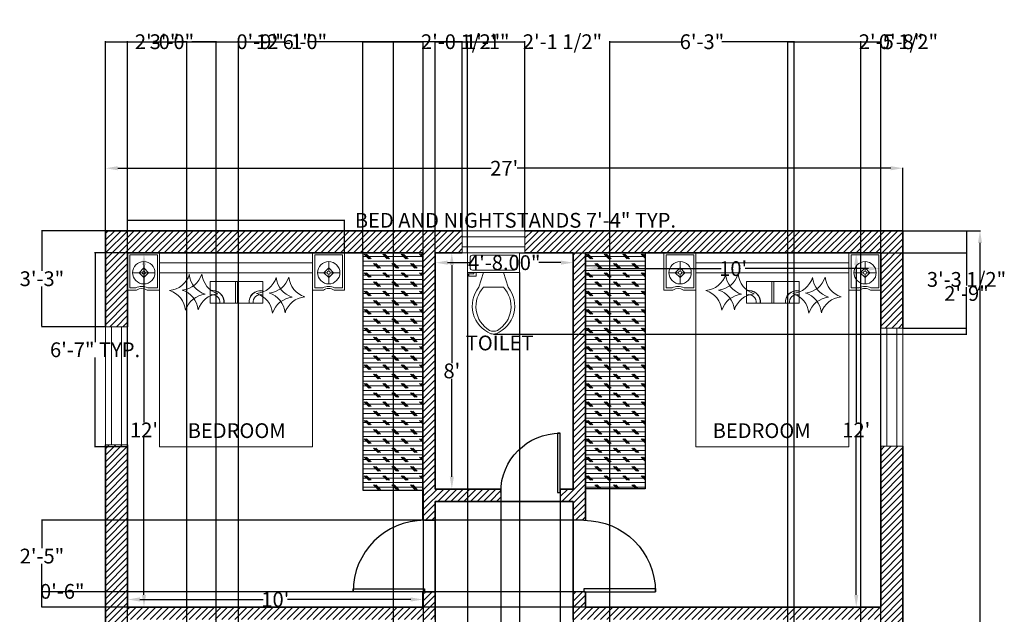
# Model space of a CAD drawing. Units: inches. Extents: x -302 to 383, y -29 to 550.
# Tile 4 of 4: x -17 to 383, y 308 to 550. Entities that reach past the tile are written whole.
import ezdxf

# ---------------------------------------------------------------- set-up
doc = ezdxf.new("R2010")
doc.units = ezdxf.units.IN
doc.header["$MEASUREMENT"] = 0
for name, color, linetype, lineweight in [('A-ANNO-DIMS', 3, 'Continuous', 18), ('A-AREA-IDEN', 2, 'Continuous', 25), ('A-DOOR', 4, 'Continuous', 25), ('A-FLOR-CASE', 7, 'Continuous', 25), ('A-FLOR-CASE-PATT', 252, 'Continuous', 13), ('A-FLOR-FIXT', 1, 'Continuous', 18), ('A-FURN', 1, 'Continuous', 18), ('A-GLAZ', 2, 'Continuous', 18), ('A-WALL', 7, 'Continuous', 35), ('A-WALL-PATT', 252, 'Continuous', 13)]:
    doc.layers.add(name, color=color, linetype=linetype, lineweight=lineweight)
doc.styles.get("Standard").update_dxf_attribs({"font": 'arial.ttf'})
doc.dimstyles.get("Standard").update_dxf_attribs({"dimtxt": 6, "dimasz": 0.18, "dimexe": 0.18, "dimexo": 0.0625, "dimgap": 0.09, "dimtad": 0, "dimtih": 1, "dimtoh": 1, "dimzin": 0, "dimdsep": 46, "dimlunit": 3, "dimtxsty": 'Standard', "dimcen": 0.09, "dimadec": 0, "dimazin": 0, "dimtfac": 1, "dimtofl": 0, "dimtmove": 0, "dimatfit": 3, "dimfxl": 1, "dimtolj": 1, "dimtzin": 0, "dimarcsym": 0})

# ---------------------------------------------------------------- blocks, each defined once
blk = doc.blocks.new('*U2')
for p, q in [((0, 0), (0, -6)), ((40, 0), (40, -6))]:
    blk.add_line(p, q)
blk.add_lwpolyline([(0, 0), (0, 40), (1.75, 40), (1.75, 0)], close=True)
blk.add_arc((0, 0), 40, 0, 90)
blk = doc.blocks.new('*U5')
for p, q in [((9.5, -6), (9.5, -2)), ((-8, -8.5), (-8, -8)), ((-7, -8), (-7, -9.5)), ((-4, -8), (-6, -14)), ((4, -8), (6, -14)), ((-10, -8.5), (-8, -8.5)), ((-10, -9.5), (-10, -8.5)), ((-7, -9.5), (-10, -9.5)), ((4, -14), (-4, -14))]:
    blk.add_line(p, q)
blk.add_lwpolyline([(10.5, -8), (10.5, 0), (-10.5, 0), (-10.5, -8)], close=True)
for points in [[(-9.5, -2), (-9.5, -6)], [(8.5, -1), (-8.5, -1)], [(-8.5, -7), (8.5, -7)]]:
    blk.add_lwpolyline(points)
for centre, radius, start, end in [((-8.62, -1.88), 0.884, 81.8699, 188.1301), ((8.62, -1.88), 0.884, 351.8699, 98.1301), ((-8.62, -6.12), 0.884, 171.8699, 278.1301), ((8.62, -6.12), 0.884, 261.8699, 8.1301), ((3.52, -21.58), 12.17, 141.4691, 247.9714), ((4.2, -21.82), 11.33, 136.3677, 238.9468), ((-3.52, -21.58), 12.17, 292.0284, 38.5307), ((-4.2, -21.82), 11.33, 301.053, 43.6321), ((0, -27.88), 4, 245.7318, 294.2682), ((0, -29), 4, 254.8605, 285.1395)]:
    blk.add_arc(centre, radius, start, end)
blk = doc.blocks.new('*D7')
at = {"layer": 'A-ANNO-DIMS', "color": 0, "lineweight": -2, "transparency": 16777216}
for p, q in [((26.7, 311.34), (26.7, 314.57)), ((31.7, 314.39), (81.8, 314.39)), ((141.7, 314.39), (91.6, 314.39)), ((146.7, 311.34), (146.7, 314.57))]:
    blk.add_line(p, q, dxfattribs=at)
at = {"layer": 'A-ANNO-DIMS', "color": 0, "transparency": 16777216}
for points in [[(31.7, 315.23), (31.7, 313.56), (26.7, 314.39)], [(141.7, 315.23), (141.7, 313.56), (146.7, 314.39)]]:
    blk.add_solid(points, dxfattribs=at)
at = {"layer": 'Defpoints', "color": 0, "transparency": 16777216}
for p in [(146.7, 314.39), (26.7, 311.27), (146.7, 311.27)]:
    blk.add_point(p, dxfattribs=at)
at = {"layer": 'A-ANNO-DIMS', "color": 0, "transparency": 16777216, "insert": (86.7, 314.39), "char_height": 6, "attachment_point": 5}
blk.add_mtext("\\A1;10'", dxfattribs=at)
blk = doc.blocks.new('*D8')
at = {"layer": 'A-ANNO-DIMS', "color": 0, "lineweight": -2, "transparency": 16777216}
for p, q in [((26.76, 455.27), (33.53, 455.27)), ((33.35, 450.27), (33.35, 386.38)), ((33.35, 316.27), (33.35, 380.17)), ((26.76, 311.27), (33.53, 311.27))]:
    blk.add_line(p, q, dxfattribs=at)
at = {"layer": 'A-ANNO-DIMS', "color": 0, "transparency": 16777216}
for points in [[(32.51, 450.27), (34.18, 450.27), (33.35, 455.27)], [(32.51, 316.27), (34.18, 316.27), (33.35, 311.27)]]:
    blk.add_solid(points, dxfattribs=at)
at = {"layer": 'Defpoints', "color": 0, "transparency": 16777216}
for p in [(26.7, 455.27), (26.7, 311.27), (33.35, 311.27)]:
    blk.add_point(p, dxfattribs=at)
at = {"layer": 'A-ANNO-DIMS', "color": 0, "transparency": 16777216, "insert": (33.35, 383.27), "char_height": 6, "attachment_point": 5}
blk.add_mtext("\\A1;12'", dxfattribs=at)
blk = doc.blocks.new('*D9')
at = {"layer": 'A-ANNO-DIMS', "color": 0, "lineweight": -2, "transparency": 16777216}
for p, q in [((151.7, 455.21), (151.7, 451.1)), ((207.7, 455.21), (207.7, 451.1)), ((156.7, 451.28), (165.69, 451.28)), ((202.7, 451.28), (193.71, 451.28))]:
    blk.add_line(p, q, dxfattribs=at)
at = {"layer": 'A-ANNO-DIMS', "color": 0, "transparency": 16777216}
for points in [[(156.7, 452.12), (156.7, 450.45), (151.7, 451.28)], [(202.7, 452.12), (202.7, 450.45), (207.7, 451.28)]]:
    blk.add_solid(points, dxfattribs=at)
at = {"layer": 'Defpoints', "color": 0, "transparency": 16777216}
for p in [(151.7, 455.27), (207.7, 455.27), (207.7, 451.28)]:
    blk.add_point(p, dxfattribs=at)
at = {"layer": 'A-ANNO-DIMS', "color": 0, "transparency": 16777216, "insert": (179.7, 451.28), "char_height": 6, "attachment_point": 5}
blk.add_mtext('\\A1;4\'-8.00"', dxfattribs=at)
blk = doc.blocks.new('*D10')
at = {"layer": 'A-ANNO-DIMS', "color": 0, "lineweight": -2, "transparency": 16777216}
for p, q in [((151.76, 455.27), (158.59, 455.27)), ((158.41, 450.27), (158.41, 410.43)), ((158.41, 364.27), (158.41, 404.12)), ((151.76, 359.27), (158.59, 359.27))]:
    blk.add_line(p, q, dxfattribs=at)
at = {"layer": 'A-ANNO-DIMS', "color": 0, "transparency": 16777216}
for points in [[(157.58, 450.27), (159.25, 450.27), (158.41, 455.27)], [(157.58, 364.27), (159.25, 364.27), (158.41, 359.27)]]:
    blk.add_solid(points, dxfattribs=at)
at = {"layer": 'Defpoints', "color": 0, "transparency": 16777216}
for p in [(151.7, 455.27), (151.7, 359.27), (158.41, 359.27)]:
    blk.add_point(p, dxfattribs=at)
at = {"layer": 'A-ANNO-DIMS', "color": 0, "transparency": 16777216, "insert": (158.41, 407.27), "char_height": 6, "attachment_point": 5}
blk.add_mtext("\\A1;8'", dxfattribs=at)
blk = doc.blocks.new('*D11')
at = {"layer": 'A-ANNO-DIMS', "color": 0, "lineweight": -2, "transparency": 16777216}
for p, q in [((212.7, 455.21), (212.7, 448.69)), ((332.7, 455.21), (332.7, 448.69)), ((217.7, 448.87), (267.8, 448.87)), ((327.7, 448.87), (277.6, 448.87))]:
    blk.add_line(p, q, dxfattribs=at)
at = {"layer": 'A-ANNO-DIMS', "color": 0, "transparency": 16777216}
for points in [[(217.7, 449.71), (217.7, 448.04), (212.7, 448.87)], [(327.7, 449.71), (327.7, 448.04), (332.7, 448.87)]]:
    blk.add_solid(points, dxfattribs=at)
at = {"layer": 'Defpoints', "color": 0, "transparency": 16777216}
for p in [(212.7, 455.27), (332.7, 455.27), (332.7, 448.87)]:
    blk.add_point(p, dxfattribs=at)
at = {"layer": 'A-ANNO-DIMS', "color": 0, "transparency": 16777216, "insert": (272.7, 448.87), "char_height": 6, "attachment_point": 5}
blk.add_mtext("\\A1;10'", dxfattribs=at)
blk = doc.blocks.new('*D12')
at = {"layer": 'A-ANNO-DIMS', "color": 0, "lineweight": -2, "transparency": 16777216}
for p, q in [((332.63, 455.27), (322.53, 455.27)), ((322.71, 450.27), (322.71, 386.38)), ((322.71, 316.27), (322.71, 380.17)), ((332.63, 311.27), (322.53, 311.27))]:
    blk.add_line(p, q, dxfattribs=at)
at = {"layer": 'A-ANNO-DIMS', "color": 0, "transparency": 16777216}
for points in [[(321.87, 450.27), (323.54, 450.27), (322.71, 455.27)], [(321.87, 316.27), (323.54, 316.27), (322.71, 311.27)]]:
    blk.add_solid(points, dxfattribs=at)
at = {"layer": 'Defpoints', "color": 0, "transparency": 16777216}
for p in [(322.71, 455.27), (332.7, 455.27), (332.7, 311.27)]:
    blk.add_point(p, dxfattribs=at)
at = {"layer": 'A-ANNO-DIMS', "color": 0, "transparency": 16777216, "insert": (322.71, 383.27), "char_height": 6, "attachment_point": 5}
blk.add_mtext("\\A1;12'", dxfattribs=at)
blk = doc.blocks.new('*D21')
at = {"layer": 'A-ANNO-DIMS', "color": 0, "lineweight": -2, "transparency": 16777216}
for p, q in [((17.7, 464.34), (17.7, 489.83)), ((22.7, 489.65), (174.46, 489.65)), ((336.7, 489.65), (184.93, 489.65)), ((341.7, 464.34), (341.7, 489.83))]:
    blk.add_line(p, q, dxfattribs=at)
at = {"layer": 'A-ANNO-DIMS', "color": 0, "transparency": 16777216}
for points in [[(22.7, 490.48), (22.7, 488.82), (17.7, 489.65)], [(336.7, 490.48), (336.7, 488.82), (341.7, 489.65)]]:
    blk.add_solid(points, dxfattribs=at)
at = {"layer": 'Defpoints', "color": 0, "transparency": 16777216}
for p in [(341.7, 489.65), (17.7, 464.27), (341.7, 464.27)]:
    blk.add_point(p, dxfattribs=at)
at = {"layer": 'A-ANNO-DIMS', "color": 0, "transparency": 16777216, "insert": (179.7, 489.65), "char_height": 6, "attachment_point": 5}
blk.add_mtext("\\A1;27'", dxfattribs=at)
blk = doc.blocks.new('*D22')
at = {"layer": 'A-ANNO-DIMS', "color": 0, "lineweight": -2, "transparency": 16777216}
for p, q in [((341.76, 464.27), (373.16, 464.27)), ((372.98, 459.27), (372.98, 245.43)), ((372.98, 25.27), (372.98, 239.12)), ((341.76, 20.27), (373.16, 20.27))]:
    blk.add_line(p, q, dxfattribs=at)
at = {"layer": 'A-ANNO-DIMS', "color": 0, "transparency": 16777216}
for points in [[(372.15, 459.27), (373.82, 459.27), (372.98, 464.27)], [(372.15, 25.27), (373.82, 25.27), (372.98, 20.27)]]:
    blk.add_solid(points, dxfattribs=at)
at = {"layer": 'Defpoints', "color": 0, "transparency": 16777216}
for p in [(341.7, 464.27), (341.7, 20.27), (372.98, 20.27)]:
    blk.add_point(p, dxfattribs=at)
at = {"layer": 'A-ANNO-DIMS', "color": 0, "transparency": 16777216, "insert": (372.98, 242.27), "char_height": 6, "attachment_point": 5}
blk.add_mtext("\\A1;37'", dxfattribs=at)
blk = doc.blocks.new('Lamp - Table')
for p, q in [((0, 7), (0, 1)), ((-1, 0), (-7, 0)), ((0, 3), (-3, 0)), ((-3, 0), (0, -3)), ((3, 0), (0, 3)), ((0, -3), (3, 0)), ((1, 0), (7, 0)), ((0, -1), (0, -7))]:
    blk.add_line(p, q)
for radius in [7, 1]:
    blk.add_circle((0, 0), radius)
blk = doc.blocks.new('BED-DOUBLE-WITH-NIGHTSTANDS')
for p, q in [((75.13, 74.72), (12.99, 74.72)), ((75.13, 70.66), (12.99, 70.66)), ((43.79, 67.17), (43.79, 58.26)), ((44.66, 67.17), (44.66, 58.26)), ((79.52, 63.66), (75.13, 63.66)), ((88.12, 63.66), (83.87, 63.66))]:
    blk.add_line(p, q)
for points in [[(3.6, 63.66), (0, 63.66), (0, 78.78), (12.99, 78.78), (12.99, 63.66), (7.94, 63.66)], [(3.36, 64.52), (0.86, 64.52), (0.86, 77.92), (12.12, 77.92), (12.12, 64.52), (8.18, 64.52)], [(88.12, 63.66), (88.12, 78.78), (75.13, 78.78), (75.13, 63.66)], [(84.11, 64.52), (87.26, 64.52), (87.26, 77.92), (76, 77.92), (76, 64.52), (79.29, 64.52)]]:
    blk.add_lwpolyline(points)
for points in [[(75.13, 78.78), (75.13, 0), (12.99, 0), (12.99, 78.78)], [(54.94, 67.17), (54.94, 58.26), (33.51, 58.26), (33.51, 67.17)]]:
    blk.add_lwpolyline(points, close=True)
for centre, radius, start, end in [((16.16, 72.79), 9.35, 275.3318, 342.5062), ((21.26, 72.97), 9.35, 275.3318, 342.5062), ((34.38, 70.85), 9.35, 185.3318, 252.5062), ((39.49, 71.03), 9.35, 185.3318, 252.5062), ((51.49, 71.58), 9.35, 275.3318, 342.5062), ((56.59, 71.76), 9.35, 275.3318, 342.5062), ((69.71, 69.64), 9.35, 185.3318, 252.5062), ((74.81, 69.82), 9.35, 185.3318, 252.5062), ((5.77, 60.2), 4.95, 60.8762, 119.1238), ((5.77, 60.2), 4.08, 57.8749, 122.1251), ((81.7, 60.2), 4.95, 60.8188, 119.1812), ((81.7, 60.2), 4.08, 57.8112, 122.1888), ((14.22, 54.57), 9.35, 5.3318, 72.5062), ((19.32, 54.75), 9.35, 5.3318, 72.5062), ((32.44, 52.63), 9.35, 95.3318, 162.5062), ((37.54, 52.81), 9.35, 95.3318, 162.5062), ((34.46, 58.75), 4.77, 354.0759, 101.4835), ((34.46, 58.75), 4.68, 353.9664, 101.698), ((34.46, 58.75), 3.04, 350.6955, 108.172), ((53.99, 58.75), 4.68, 78.302, 186.0336), ((53.99, 58.75), 4.59, 78.302, 186.0336), ((53.99, 58.75), 3.04, 71.828, 189.3045), ((49.55, 53.36), 9.35, 5.3318, 72.5062), ((54.65, 53.54), 9.35, 5.3318, 72.5062), ((67.77, 51.42), 9.35, 95.3318, 162.5062), ((72.87, 51.6), 9.35, 95.3318, 162.5062)]:
    blk.add_arc(centre, radius, start, end)
at = {"xscale": 0.6492676873640278, "yscale": 0.6492676873640278, "zscale": 0.6492676873640278, "rotation": 270}
for p in [(6.58, 70.7), (81.7, 70.7)]:
    blk.add_blockref('Lamp - Table', p, dxfattribs=at)
blk = doc.blocks.new('WIN-48IN')
blk.add_lwpolyline([(0, 9), (48, 9), (48, 0), (0, 0)], close=True)
for points in [[(0, 6.5), (48, 6.5)], [(0, 2.5), (48, 2.5)]]:
    blk.add_lwpolyline(points)
blk = doc.blocks.new('*D31')
at = {"layer": 'A-ANNO-DIMS', "color": 0, "lineweight": -2, "transparency": 16777216}
for p, q in [((26.7, 455.34), (26.7, 468.67)), ((26.88, 468.49), (114.64, 468.49)), ((114.82, 455.34), (114.82, 468.67)), ((114.82, 468.49), (115, 468.49))]:
    blk.add_line(p, q, dxfattribs=at)
at = {"layer": 'A-ANNO-DIMS', "color": 0, "transparency": 16777216}
for points in [[(26.88, 468.52), (26.88, 468.46), (26.7, 468.49)], [(114.64, 468.52), (114.64, 468.46), (114.82, 468.49)]]:
    blk.add_solid(points, dxfattribs=at)
at = {"layer": 'Defpoints', "color": 0, "transparency": 16777216}
for p in [(114.82, 468.49), (26.7, 455.27), (114.82, 455.27)]:
    blk.add_point(p, dxfattribs=at)
at = {"layer": 'A-ANNO-DIMS', "color": 0, "transparency": 16777216, "insert": (184.24, 468.49), "char_height": 6, "attachment_point": 5}
blk.add_mtext('\\A1;BED AND NIGHTSTANDS 7\'-4" TYP.', dxfattribs=at)
blk = doc.blocks.new('*D32')
at = {"layer": 'A-ANNO-DIMS', "color": 0, "lineweight": -2, "transparency": 16777216}
for p, q in [((26.63, 455.27), (13.3, 455.27)), ((13.48, 455.09), (13.48, 419.03)), ((13.48, 376.67), (13.48, 412.73)), ((26.63, 376.49), (13.3, 376.49))]:
    blk.add_line(p, q, dxfattribs=at)
at = {"layer": 'A-ANNO-DIMS', "color": 0, "transparency": 16777216}
for points in [[(13.45, 455.09), (13.51, 455.09), (13.48, 455.27)], [(13.45, 376.67), (13.51, 376.67), (13.48, 376.49)]]:
    blk.add_solid(points, dxfattribs=at)
at = {"layer": 'Defpoints', "color": 0, "transparency": 16777216}
for p in [(13.48, 455.27), (26.7, 455.27), (26.7, 376.49)]:
    blk.add_point(p, dxfattribs=at)
at = {"layer": 'A-ANNO-DIMS', "color": 0, "transparency": 16777216, "insert": (13.48, 415.88), "char_height": 6, "attachment_point": 5}
blk.add_mtext('\\A1;6\'-7" TYP.', dxfattribs=at)
blk = doc.blocks.new('*D44')
at = {"layer": 'A-ANNO-DIMS', "color": 0, "lineweight": -2, "transparency": 16777216}
for p, q in [((17.63, 464.27), (-8.28, 464.27)), ((-8.1, 464.09), (-8.1, 447.9)), ((-8.1, 425.4), (-8.1, 441.59)), ((17.63, 425.22), (-8.28, 425.22))]:
    blk.add_line(p, q, dxfattribs=at)
at = {"layer": 'A-ANNO-DIMS', "color": 0, "transparency": 16777216}
for points in [[(-8.13, 464.09), (-8.07, 464.09), (-8.1, 464.27)], [(-8.13, 425.4), (-8.07, 425.4), (-8.1, 425.22)]]:
    blk.add_solid(points, dxfattribs=at)
at = {"layer": 'Defpoints', "color": 0, "transparency": 16777216}
for p in [(-8.1, 464.27), (17.7, 464.27), (17.7, 425.22)]:
    blk.add_point(p, dxfattribs=at)
at = {"layer": 'A-ANNO-DIMS', "color": 0, "transparency": 16777216, "insert": (-8.1, 444.75), "char_height": 6, "attachment_point": 5}
blk.add_mtext('\\A1;3\'-3"', dxfattribs=at)
blk = doc.blocks.new('*D46')
at = {"layer": 'A-ANNO-DIMS', "color": 0, "lineweight": -2, "transparency": 16777216}
for p, q in [((341.76, 464.27), (367.68, 464.27)), ((367.5, 464.09), (367.5, 447.67)), ((367.5, 424.85), (367.5, 441.28)), ((341.76, 424.67), (367.68, 424.67))]:
    blk.add_line(p, q, dxfattribs=at)
at = {"layer": 'A-ANNO-DIMS', "color": 0, "transparency": 16777216}
for points in [[(367.47, 464.09), (367.53, 464.09), (367.5, 464.27)], [(367.47, 424.85), (367.53, 424.85), (367.5, 424.67)]]:
    blk.add_solid(points, dxfattribs=at)
at = {"layer": 'Defpoints', "color": 0, "transparency": 16777216}
for p in [(341.7, 464.27), (367.5, 464.27), (341.7, 424.67)]:
    blk.add_point(p, dxfattribs=at)
at = {"layer": 'A-ANNO-DIMS', "color": 0, "transparency": 16777216, "insert": (367.5, 444.47), "char_height": 6, "attachment_point": 5}
blk.add_mtext('\\A1;3\'-3 1/2"', dxfattribs=at)
blk = doc.blocks.new('*D47')
at = {"layer": 'A-ANNO-DIMS', "color": 0, "lineweight": -2, "transparency": 16777216}
for p, q in [((162.63, 464.34), (162.63, 541.25)), ((162.81, 541.07), (187.9, 541.07)), ((188.08, 464.34), (188.08, 541.25)), ((188.08, 541.07), (188.26, 541.07))]:
    blk.add_line(p, q, dxfattribs=at)
at = {"layer": 'A-ANNO-DIMS', "color": 0, "transparency": 16777216}
for points in [[(162.81, 541.1), (162.81, 541.04), (162.63, 541.07)], [(187.9, 541.1), (187.9, 541.04), (188.08, 541.07)]]:
    blk.add_solid(points, dxfattribs=at)
at = {"layer": 'Defpoints', "color": 0, "transparency": 16777216}
for p in [(188.08, 541.07), (162.63, 464.27), (188.08, 464.27)]:
    blk.add_point(p, dxfattribs=at)
at = {"layer": 'A-ANNO-DIMS', "color": 0, "transparency": 16777216, "insert": (203.36, 541.07), "char_height": 6, "attachment_point": 5}
blk.add_mtext('\\A1;2\'-1 1/2"', dxfattribs=at)
blk = doc.blocks.new('*D48')
at = {"layer": 'A-ANNO-DIMS', "color": 0, "lineweight": -2, "transparency": 16777216}
for p, q in [((17.7, 464.34), (17.7, 541.25)), ((17.88, 541.07), (80.05, 541.07)), ((162.45, 541.07), (100.28, 541.07)), ((162.63, 464.34), (162.63, 541.25))]:
    blk.add_line(p, q, dxfattribs=at)
at = {"layer": 'A-ANNO-DIMS', "color": 0, "transparency": 16777216}
for points in [[(17.88, 541.1), (17.88, 541.04), (17.7, 541.07)], [(162.45, 541.1), (162.45, 541.04), (162.63, 541.07)]]:
    blk.add_solid(points, dxfattribs=at)
at = {"layer": 'Defpoints', "color": 0, "transparency": 16777216}
for p in [(162.63, 541.07), (17.7, 464.27), (162.63, 464.27)]:
    blk.add_point(p, dxfattribs=at)
at = {"layer": 'A-ANNO-DIMS', "color": 0, "transparency": 16777216, "insert": (90.17, 541.07), "char_height": 6, "attachment_point": 5}
blk.add_mtext('\\A1;12\'-1"', dxfattribs=at)
blk = doc.blocks.new('*D49')
at = {"layer": 'A-ANNO-DIMS', "color": 0, "lineweight": -2, "transparency": 16777216}
for p, q in [((207.63, 346.57), (-8.28, 346.57)), ((-8.1, 346.39), (-8.1, 335.19)), ((-8.1, 317.69), (-8.1, 328.89)), ((207.63, 317.51), (-8.28, 317.51))]:
    blk.add_line(p, q, dxfattribs=at)
at = {"layer": 'A-ANNO-DIMS', "color": 0, "transparency": 16777216}
for points in [[(-8.13, 346.39), (-8.07, 346.39), (-8.1, 346.57)], [(-8.13, 317.69), (-8.07, 317.69), (-8.1, 317.51)]]:
    blk.add_solid(points, dxfattribs=at)
at = {"layer": 'Defpoints', "color": 0, "transparency": 16777216}
for p in [(-8.1, 346.57), (207.7, 346.57), (207.7, 317.51)]:
    blk.add_point(p, dxfattribs=at)
at = {"layer": 'A-ANNO-DIMS', "color": 0, "transparency": 16777216, "insert": (-8.1, 332.04), "char_height": 6, "attachment_point": 5}
blk.add_mtext('\\A1;2\'-5"', dxfattribs=at)
blk = doc.blocks.new('*D50')
at = {"layer": 'A-ANNO-DIMS', "color": 0, "lineweight": -2, "transparency": 16777216}
for p, q in [((178.34, 359.21), (178.34, -5.71)), ((202.4, 359.21), (202.4, -5.71)), ((178.52, -5.53), (182.25, -5.53)), ((202.22, -5.53), (198.48, -5.53))]:
    blk.add_line(p, q, dxfattribs=at)
at = {"layer": 'A-ANNO-DIMS', "color": 0, "transparency": 16777216}
for points in [[(178.52, -5.5), (178.52, -5.56), (178.34, -5.53)], [(202.22, -5.5), (202.22, -5.56), (202.4, -5.53)]]:
    blk.add_solid(points, dxfattribs=at)
at = {"layer": 'Defpoints', "color": 0, "transparency": 16777216}
for p in [(178.34, 359.27), (202.4, 359.27), (202.4, -5.53)]:
    blk.add_point(p, dxfattribs=at)
at = {"layer": 'A-ANNO-DIMS', "color": 0, "transparency": 16777216, "insert": (190.37, -5.53), "char_height": 6, "attachment_point": 5}
blk.add_mtext('\\A1;2\'-0"', dxfattribs=at)
blk = doc.blocks.new('*D53')
at = {"layer": 'A-ANNO-DIMS', "color": 0, "lineweight": -2, "transparency": 16777216}
for p, q in [((294.85, 149.34), (294.85, 541.25)), ((295.03, 541.07), (324.38, 541.07)), ((324.56, 149.34), (324.56, 541.25)), ((324.56, 541.07), (324.74, 541.07))]:
    blk.add_line(p, q, dxfattribs=at)
at = {"layer": 'A-ANNO-DIMS', "color": 0, "transparency": 16777216}
for points in [[(295.03, 541.1), (295.03, 541.04), (294.85, 541.07)], [(324.38, 541.1), (324.38, 541.04), (324.56, 541.07)]]:
    blk.add_solid(points, dxfattribs=at)
at = {"layer": 'Defpoints', "color": 0, "transparency": 16777216}
for p in [(324.56, 541.07), (294.85, 149.27), (324.56, 149.27)]:
    blk.add_point(p, dxfattribs=at)
at = {"layer": 'A-ANNO-DIMS', "color": 0, "transparency": 16777216, "insert": (339.85, 541.07), "char_height": 6, "attachment_point": 5}
blk.add_mtext('\\A1;2\'-5 1/2"', dxfattribs=at)
blk = doc.blocks.new('*D54')
at = {"layer": 'A-ANNO-DIMS', "color": 0, "lineweight": -2, "transparency": 16777216}
for p, q in [((26.7, 226.34), (26.7, 541.25)), ((26.88, 541.07), (36.63, 541.07)), ((62.52, 541.07), (52.76, 541.07)), ((62.7, 226.34), (62.7, 541.25))]:
    blk.add_line(p, q, dxfattribs=at)
at = {"layer": 'A-ANNO-DIMS', "color": 0, "transparency": 16777216}
for points in [[(26.88, 541.1), (26.88, 541.04), (26.7, 541.07)], [(62.52, 541.1), (62.52, 541.04), (62.7, 541.07)]]:
    blk.add_solid(points, dxfattribs=at)
at = {"layer": 'Defpoints', "color": 0, "transparency": 16777216}
for p in [(62.7, 541.07), (26.7, 226.27), (62.7, 226.27)]:
    blk.add_point(p, dxfattribs=at)
at = {"layer": 'A-ANNO-DIMS', "color": 0, "transparency": 16777216, "insert": (44.7, 541.07), "char_height": 6, "attachment_point": 5}
blk.add_mtext('\\A1;3\'-0"', dxfattribs=at)
blk = doc.blocks.new('*D55')
at = {"layer": 'A-ANNO-DIMS', "color": 0, "lineweight": -2, "transparency": 16777216}
for p, q in [((62.7, 226.34), (62.7, 541.25)), ((62.88, 541.07), (90.62, 541.07)), ((134.52, 541.07), (106.78, 541.07)), ((134.7, 226.34), (134.7, 541.25))]:
    blk.add_line(p, q, dxfattribs=at)
at = {"layer": 'A-ANNO-DIMS', "color": 0, "transparency": 16777216}
for points in [[(62.88, 541.1), (62.88, 541.04), (62.7, 541.07)], [(134.52, 541.1), (134.52, 541.04), (134.7, 541.07)]]:
    blk.add_solid(points, dxfattribs=at)
at = {"layer": 'Defpoints', "color": 0, "transparency": 16777216}
for p in [(134.7, 541.07), (62.7, 226.27), (134.7, 226.27)]:
    blk.add_point(p, dxfattribs=at)
at = {"layer": 'A-ANNO-DIMS', "color": 0, "transparency": 16777216, "insert": (98.7, 541.07), "char_height": 6, "attachment_point": 5}
blk.add_mtext('\\A1;6\'-0"', dxfattribs=at)
blk = doc.blocks.new('*D57')
at = {"layer": 'A-ANNO-DIMS', "color": 0, "lineweight": -2, "transparency": 16777216}
for p, q in [((26.7, 158.79), (26.7, 541.25)), ((26.88, 541.07), (30.58, 541.07)), ((50.52, 541.07), (46.81, 541.07)), ((50.7, 158.79), (50.7, 541.25))]:
    blk.add_line(p, q, dxfattribs=at)
at = {"layer": 'A-ANNO-DIMS', "color": 0, "transparency": 16777216}
for points in [[(26.88, 541.1), (26.88, 541.04), (26.7, 541.07)], [(50.52, 541.1), (50.52, 541.04), (50.7, 541.07)]]:
    blk.add_solid(points, dxfattribs=at)
at = {"layer": 'Defpoints', "color": 0, "transparency": 16777216}
for p in [(50.7, 541.07), (26.7, 158.73), (50.7, 158.73)]:
    blk.add_point(p, dxfattribs=at)
at = {"layer": 'A-ANNO-DIMS', "color": 0, "transparency": 16777216, "insert": (38.7, 541.07), "char_height": 6, "attachment_point": 5}
blk.add_mtext('\\A1;2\'-0"', dxfattribs=at)
blk = doc.blocks.new('*D59')
at = {"layer": 'A-ANNO-DIMS', "color": 0, "lineweight": -2, "transparency": 16777216}
for p, q in [((122.2, 455.34), (122.2, 541.25)), ((122.38, 541.07), (146.52, 541.07)), ((146.7, 455.34), (146.7, 541.25)), ((146.7, 541.07), (146.88, 541.07))]:
    blk.add_line(p, q, dxfattribs=at)
at = {"layer": 'A-ANNO-DIMS', "color": 0, "transparency": 16777216}
for points in [[(122.38, 541.1), (122.38, 541.04), (122.2, 541.07)], [(146.52, 541.1), (146.52, 541.04), (146.7, 541.07)]]:
    blk.add_solid(points, dxfattribs=at)
at = {"layer": 'Defpoints', "color": 0, "transparency": 16777216}
for p in [(146.7, 541.07), (122.2, 455.27), (146.7, 455.27)]:
    blk.add_point(p, dxfattribs=at)
at = {"layer": 'A-ANNO-DIMS', "color": 0, "transparency": 16777216, "insert": (161.98, 541.07), "char_height": 6, "attachment_point": 5}
blk.add_mtext('\\A1;2\'-0 1/2"', dxfattribs=at)
blk = doc.blocks.new('*D60')
at = {"layer": 'A-ANNO-DIMS', "color": 0, "lineweight": -2, "transparency": 16777216}
for p, q in [((164.84, 447.21), (164.84, -5.71)), ((185.84, 447.21), (185.84, -5.71)), ((165.02, -5.53), (167.56, -5.53)), ((185.66, -5.53), (183.12, -5.53))]:
    blk.add_line(p, q, dxfattribs=at)
at = {"layer": 'A-ANNO-DIMS', "color": 0, "transparency": 16777216}
for points in [[(165.02, -5.5), (165.02, -5.56), (164.84, -5.53)], [(185.66, -5.5), (185.66, -5.56), (185.84, -5.53)]]:
    blk.add_solid(points, dxfattribs=at)
at = {"layer": 'Defpoints', "color": 0, "transparency": 16777216}
for p in [(164.84, 447.27), (185.84, 447.27), (185.84, -5.53)]:
    blk.add_point(p, dxfattribs=at)
at = {"layer": 'A-ANNO-DIMS', "color": 0, "transparency": 16777216, "insert": (175.34, -5.53), "char_height": 6, "attachment_point": 5}
blk.add_mtext('\\A1;1\'-9"', dxfattribs=at)
blk = doc.blocks.new('*D61')
at = {"layer": 'A-ANNO-DIMS', "color": 0, "lineweight": -2, "transparency": 16777216}
for p, q in [((185.9, 455.27), (367.68, 455.27)), ((367.5, 455.09), (367.5, 441.93)), ((367.5, 422.45), (367.5, 435.62)), ((175.4, 422.27), (367.68, 422.27))]:
    blk.add_line(p, q, dxfattribs=at)
at = {"layer": 'A-ANNO-DIMS', "color": 0, "transparency": 16777216}
for points in [[(367.47, 455.09), (367.53, 455.09), (367.5, 455.27)], [(367.47, 422.45), (367.53, 422.45), (367.5, 422.27)]]:
    blk.add_solid(points, dxfattribs=at)
at = {"layer": 'Defpoints', "color": 0, "transparency": 16777216}
for p in [(185.84, 455.27), (175.34, 422.27), (367.5, 422.27)]:
    blk.add_point(p, dxfattribs=at)
at = {"layer": 'A-ANNO-DIMS', "color": 0, "transparency": 16777216, "insert": (367.5, 438.77), "char_height": 6, "attachment_point": 5}
blk.add_mtext('\\A1;2\'-9"', dxfattribs=at)
blk = doc.blocks.new('*D62')
at = {"layer": 'A-ANNO-DIMS', "color": 0, "lineweight": -2, "transparency": 16777216}
for p, q in [((222.62, 298.67), (222.62, 541.25)), ((222.8, 541.07), (251.95, 541.07)), ((297.27, 541.07), (268.11, 541.07)), ((297.45, 298.67), (297.45, 541.25))]:
    blk.add_line(p, q, dxfattribs=at)
at = {"layer": 'A-ANNO-DIMS', "color": 0, "transparency": 16777216}
for points in [[(222.8, 541.1), (222.8, 541.04), (222.62, 541.07)], [(297.27, 541.1), (297.27, 541.04), (297.45, 541.07)]]:
    blk.add_solid(points, dxfattribs=at)
at = {"layer": 'Defpoints', "color": 0, "transparency": 16777216}
for p in [(297.45, 541.07), (222.62, 298.61), (297.45, 298.61)]:
    blk.add_point(p, dxfattribs=at)
at = {"layer": 'A-ANNO-DIMS', "color": 0, "transparency": 16777216, "insert": (260.03, 541.07), "char_height": 6, "attachment_point": 5}
blk.add_mtext('\\A1;6\'-3"', dxfattribs=at)
blk = doc.blocks.new('*D68')
at = {"layer": 'A-ANNO-DIMS', "color": 0, "lineweight": -2, "transparency": 16777216}
for p, q in [((62.7, 268.34), (62.7, 541.25)), ((62.88, 541.07), (71.52, 541.07)), ((71.7, 264.34), (71.7, 541.25)), ((71.7, 541.07), (71.88, 541.07))]:
    blk.add_line(p, q, dxfattribs=at)
at = {"layer": 'A-ANNO-DIMS', "color": 0, "transparency": 16777216}
for points in [[(62.88, 541.1), (62.88, 541.04), (62.7, 541.07)], [(71.52, 541.1), (71.52, 541.04), (71.7, 541.07)]]:
    blk.add_solid(points, dxfattribs=at)
at = {"layer": 'Defpoints', "color": 0, "transparency": 16777216}
for p in [(71.7, 541.07), (62.7, 268.27), (71.7, 264.27)]:
    blk.add_point(p, dxfattribs=at)
at = {"layer": 'A-ANNO-DIMS', "color": 0, "transparency": 16777216, "insert": (79.94, 541.07), "char_height": 6, "attachment_point": 5}
blk.add_mtext('\\A1;0\'-9"', dxfattribs=at)
blk = doc.blocks.new('*D71')
at = {"layer": 'A-ANNO-DIMS', "color": 0, "lineweight": -2, "transparency": 16777216}
for p, q in [((146.7, 358.81), (146.7, -5.71)), ((151.7, 354.21), (151.7, -5.71)), ((146.88, -5.53), (151.52, -5.53)), ((151.7, -5.53), (151.88, -5.53))]:
    blk.add_line(p, q, dxfattribs=at)
at = {"layer": 'A-ANNO-DIMS', "color": 0, "transparency": 16777216}
for points in [[(146.88, -5.5), (146.88, -5.56), (146.7, -5.53)], [(151.52, -5.5), (151.52, -5.56), (151.7, -5.53)]]:
    blk.add_solid(points, dxfattribs=at)
at = {"layer": 'Defpoints', "color": 0, "transparency": 16777216}
for p in [(146.7, 358.87), (151.7, 354.27), (151.7, -5.53)]:
    blk.add_point(p, dxfattribs=at)
at = {"layer": 'A-ANNO-DIMS', "color": 0, "transparency": 16777216, "insert": (159.94, -5.53), "char_height": 6, "attachment_point": 5}
blk.add_mtext('\\A1;0\'-5"', dxfattribs=at)
blk = doc.blocks.new('*D72')
at = {"layer": 'A-ANNO-DIMS', "color": 0, "lineweight": -2, "transparency": 16777216}
for p, q in [((202.4, 354.21), (202.4, -5.71)), ((207.7, 354.21), (207.7, -5.71)), ((202.58, -5.53), (207.52, -5.53)), ((207.7, -5.53), (207.88, -5.53))]:
    blk.add_line(p, q, dxfattribs=at)
at = {"layer": 'A-ANNO-DIMS', "color": 0, "transparency": 16777216}
for points in [[(202.58, -5.5), (202.58, -5.56), (202.4, -5.53)], [(207.52, -5.5), (207.52, -5.56), (207.7, -5.53)]]:
    blk.add_solid(points, dxfattribs=at)
at = {"layer": 'Defpoints', "color": 0, "transparency": 16777216}
for p in [(202.4, 354.27), (207.7, 354.27), (207.7, -5.53)]:
    blk.add_point(p, dxfattribs=at)
at = {"layer": 'A-ANNO-DIMS', "color": 0, "transparency": 16777216, "insert": (222.93, -5.53), "char_height": 6, "attachment_point": 5}
blk.add_mtext('\\A1;0\'-5 1/2"', dxfattribs=at)
blk = doc.blocks.new('*D73')
at = {"layer": 'A-ANNO-DIMS', "color": 0, "lineweight": -2, "transparency": 16777216}
for p, q in [((151.7, 455.34), (151.7, 541.25)), ((151.88, 541.07), (164.66, 541.07)), ((164.84, 455.34), (164.84, 541.25)), ((164.84, 541.07), (165.02, 541.07))]:
    blk.add_line(p, q, dxfattribs=at)
at = {"layer": 'A-ANNO-DIMS', "color": 0, "transparency": 16777216}
for points in [[(151.88, 541.1), (151.88, 541.04), (151.7, 541.07)], [(164.66, 541.1), (164.66, 541.04), (164.84, 541.07)]]:
    blk.add_solid(points, dxfattribs=at)
at = {"layer": 'Defpoints', "color": 0, "transparency": 16777216}
for p in [(164.84, 541.07), (151.7, 455.27), (164.84, 455.27)]:
    blk.add_point(p, dxfattribs=at)
at = {"layer": 'A-ANNO-DIMS', "color": 0, "transparency": 16777216, "insert": (172.8, 541.07), "char_height": 6, "attachment_point": 5}
blk.add_mtext('\\A1;1\'-1"', dxfattribs=at)
blk = doc.blocks.new('*D74')
at = {"layer": 'A-ANNO-DIMS', "color": 0, "lineweight": -2, "transparency": 16777216}
for p, q in [((324.56, 149.34), (324.56, 541.25)), ((324.74, 541.07), (332.52, 541.07)), ((332.7, 149.34), (332.7, 541.25)), ((332.7, 541.07), (332.88, 541.07))]:
    blk.add_line(p, q, dxfattribs=at)
at = {"layer": 'A-ANNO-DIMS', "color": 0, "transparency": 16777216}
for points in [[(324.74, 541.1), (324.74, 541.04), (324.56, 541.07)], [(332.52, 541.1), (332.52, 541.04), (332.7, 541.07)]]:
    blk.add_solid(points, dxfattribs=at)
at = {"layer": 'Defpoints', "color": 0, "transparency": 16777216}
for p in [(332.7, 541.07), (324.56, 149.27), (332.7, 149.27)]:
    blk.add_point(p, dxfattribs=at)
at = {"layer": 'A-ANNO-DIMS', "color": 0, "transparency": 16777216, "insert": (340.94, 541.07), "char_height": 6, "attachment_point": 5}
blk.add_mtext('\\A1;0\'-8"', dxfattribs=at)
blk = doc.blocks.new('*D75')
at = {"layer": 'A-ANNO-DIMS', "color": 0, "lineweight": -2, "transparency": 16777216}
for p, q in [((212.63, 317.51), (-8.28, 317.51)), ((-8.1, 317.51), (-8.1, 317.69)), ((-8.1, 317.69), (-7.92, 317.69)), ((-8.1, 311.45), (-8.1, 317.33)), ((212.63, 311.27), (-8.28, 311.27))]:
    blk.add_line(p, q, dxfattribs=at)
at = {"layer": 'A-ANNO-DIMS', "color": 0, "transparency": 16777216}
for points in [[(-8.13, 317.33), (-8.07, 317.33), (-8.1, 317.51)], [(-8.13, 311.45), (-8.07, 311.45), (-8.1, 311.27)]]:
    blk.add_solid(points, dxfattribs=at)
at = {"layer": 'Defpoints', "color": 0, "transparency": 16777216}
for p in [(-8.1, 317.51), (212.7, 317.51), (212.7, 311.27)]:
    blk.add_point(p, dxfattribs=at)
at = {"layer": 'A-ANNO-DIMS', "color": 0, "transparency": 16777216, "insert": (0.14, 317.69), "char_height": 6, "attachment_point": 5}
blk.add_mtext('\\A1;0\'-6"', dxfattribs=at)

msp = doc.modelspace()

# ---------------------------------------------------------------- hatches: boundary and pattern name
at = {"layer": 'A-FLOR-CASE-PATT'}
h = msp.add_hatch(dxfattribs=at)
h.set_pattern_fill('CORK', color=256, scale=15)
h.set_pattern_definition([(0, (0, 0), (0, 1.875), []), (135, (0.9375, -0.9375), (-3.75, -3.75), [2.65165, -2.65165]), (135, (1.406, -0.9375), (-3.75, -3.75), [2.65165, -2.65165]), (135, (1.875, -0.9375), (-3.75, -3.75), [2.65165, -2.65165])])
h.paths.add_polyline_path([(146.697, 455.273), (122.2, 455.273), (122.2, 358.869), (146.697, 358.869)])
h.paths.add_polyline_path([(236.952, 455.273), (212.697, 455.273), (212.697, 359.383), (236.952, 359.383)])
at = {"layer": 'A-WALL-PATT'}
h = msp.add_hatch(dxfattribs=at)
h.set_pattern_fill('ANSI31', color=256, scale=15)
h.paths.add_polyline_path([(201.697, 29.273), (187.202, 29.273), (187.202, 20.273), (251.158, 20.273), (251.158, 29.273), (206.697, 29.273), (206.697, 149.273), (294.846, 149.273, -0.0045588), (294.841, 149.815), (294.841, 154.273), (201.697, 154.273), (201.697, 130.273), (190.923, 130.273), (190.923, 125.273), (201.697, 125.273)])
h.paths.add_polyline_path([(341.697, 154.273), (332.697, 154.273), (324.561, 154.273), (324.561, 149.815), (324.561, 149.273), (332.697, 149.273), (332.697, 29.273), (299.158, 29.273), (299.158, 20.273), (341.697, 20.273)])
h.paths.add_polyline_path([(75.47, 20.273), (75.47, 29.273), (26.697, 29.273), (26.697, 89.142), (17.697, 89.142), (17.697, 20.273)])
h.paths.add_polyline_path([(26.697, 221.273), (146.697, 221.273), (146.697, 217.323), (147.147, 217.323), (151.697, 217.323), (151.697, 226.273), (26.697, 226.273), (26.697, 248.984), (17.697, 248.984), (17.697, 137.142), (26.697, 137.142)])
h.paths.add_polyline_path([(17.697, 284.934), (26.697, 284.934), (26.697, 306.273), (151.697, 306.273), (151.697, 317.511), (147.338, 317.511), (146.697, 317.511), (146.697, 311.273), (26.697, 311.273), (26.697, 377.22), (17.697, 377.22)])
h.paths.add_polyline_path([(341.697, 376.674), (332.697, 376.674), (332.697, 311.273), (212.697, 311.273), (212.697, 317.511), (212.055, 317.511), (207.697, 317.511), (207.697, 306.273), (332.697, 306.273), (332.697, 214.273), (341.697, 214.273)])
h.paths.add_polyline_path([(207.697, 455.273), (207.697, 359.273), (202.395, 359.273), (202.395, 357.888), (202.395, 354.273), (207.697, 354.273), (207.697, 346.57), (212.055, 346.57, -0.0055163), (212.697, 346.563), (212.697, 455.273), (332.697, 455.273), (332.697, 424.674), (341.697, 424.674), (341.697, 464.273), (188.075, 464.273), (188.075, 455.273)])
h.paths.add_polyline_path([(17.697, 464.273), (17.697, 425.22), (26.697, 425.22), (26.697, 455.273), (146.697, 455.273), (146.697, 346.563, -0.0055163), (147.338, 346.57), (151.697, 346.57), (151.697, 354.273), (178.3, 354.273), (178.3, 357.888, -0.0143868), (178.34, 359.273), (151.697, 359.273), (151.697, 455.273), (162.634, 455.273), (162.634, 464.273)])

# ---------------------------------------------------------------- linework, layer by layer
at = {"layer": 'A-FLOR-CASE'}
for points in [[(146.697, 455.273), (122.2, 455.273), (122.2, 358.869), (146.697, 358.869)], [(212.697, 455.273), (236.952, 455.273), (236.952, 359.383), (212.697, 359.383)]]:
    msp.add_lwpolyline(points, close=True, dxfattribs=at)
at = {"layer": 'A-GLAZ'}
msp.add_lwpolyline([(162.634, 464.273), (188.075, 464.273), (188.075, 455.273), (162.634, 455.273)], close=True, dxfattribs=at)
for points in [[(188.075, 461.773), (162.634, 461.773)], [(188.075, 457.773), (162.634, 457.773)]]:
    msp.add_lwpolyline(points, dxfattribs=at)
at = {"layer": 'A-WALL'}
for points in [[(162.634, 464.273), (17.697, 464.273), (17.697, 425.22)], [(341.697, 424.674), (341.697, 464.273), (188.075, 464.273)], [(26.697, 455.273), (26.697, 425.22)], [(146.697, 455.273), (26.697, 455.273)], [(146.697, 455.273), (146.697, 346.563)], [(151.697, 455.273), (151.697, 359.273)], [(162.634, 455.273), (151.697, 455.273)], [(207.697, 455.273), (188.075, 455.273)], [(207.697, 359.273), (207.697, 455.273)], [(332.697, 455.273), (212.697, 455.273)], [(212.697, 346.563), (212.697, 455.273)], [(332.697, 424.674), (332.697, 455.273)], [(17.697, 377.22), (17.697, 284.934)], [(26.697, 377.22), (26.697, 311.273)], [(332.697, 311.273), (332.697, 376.674)], [(341.697, 214.273), (341.697, 376.674)], [(178.34, 359.273), (151.697, 359.273)], [(207.697, 359.273), (202.395, 359.273)], [(207.697, 354.273), (151.697, 354.273)], [(151.697, 354.273), (151.697, 306.273)], [(207.697, 306.273), (207.697, 354.273)], [(146.697, 317.511), (146.697, 311.273)], [(212.697, 311.273), (212.697, 317.511)], [(146.697, 311.273), (26.697, 311.273)], [(332.697, 311.273), (212.697, 311.273)]]:
    msp.add_lwpolyline(points, dxfattribs=at)

# ---------------------------------------------------------------- block references
at = {"layer": 'A-DOOR', "xscale": -0.6023763508036813, "yscale": 0.6023763508036813, "zscale": 0.6023763508036813}
msp.add_blockref('*U2', (202.395, 357.888), dxfattribs=at)
at = {"layer": 'A-DOOR', "yscale": 0.7264772032696051, "zscale": 0.7264772032696051}
for p, xscale, rotation in [((147.338, 317.511), 0.7264772032696051, 90.00000000000003), ((212.055, 317.511), -0.7264772032696051, 270)]:
    msp.add_blockref('*U2', p, dxfattribs=dict(at, xscale=xscale, rotation=rotation))
at = {"layer": 'A-FLOR-FIXT'}
msp.add_blockref('*U5', (175.341, 455.273), dxfattribs=at)
at = {"layer": 'A-FURN'}
for p in [(26.697, 376.489), (244.577, 376.489)]:
    msp.add_blockref('BED-DOUBLE-WITH-NIGHTSTANDS', p, dxfattribs=at)
at = {"layer": 'A-GLAZ', "extrusion": (0, 0, -1), "zscale": -1}
for p, rotation in [((-26.697, 425.22), 270), ((-341.697, 424.674), 270.0000000000001)]:
    msp.add_blockref('WIN-48IN', p, dxfattribs=dict(at, rotation=rotation))

# ---------------------------------------------------------------- texts
at = {"layer": 'A-AREA-IDEN', "char_height": 6, "attachment_point": 1}
for s, insert in [('{TOILET}', (164.064, 421.637)), ('{BEDROOM}', (51.094, 386.001)), ('{BEDROOM}', (264.357, 386.001))]:
    msp.add_mtext_dynamic_manual_height_columns(s, width=101.54109, gutter_width=1, heights=[0], dxfattribs=dict(at, insert=insert))

# ---------------------------------------------------------------- dimensions: what is measured, and where the dimension line sits
at = {"layer": 'A-ANNO-DIMS'}
for base, p1, p2, override, picture, middle in [((146.697, 541.073), (122.2, 455.273), (146.697, 455.273), {"dimdec": 1, "dimlfac": 1, "dimrnd": 0, "dimzin": 1, "dimdsep": 46, "dimlunit": 4, "dimfrac": 2}, '*D59', (161.983, 541.073)), ((188.075, 541.073), (162.634, 464.273), (188.075, 464.273), {"dimdec": 1, "dimlfac": 1, "dimrnd": 0, "dimzin": 1, "dimdsep": 46, "dimlunit": 4, "dimfrac": 2}, '*D47', (203.362, 541.073)), ((324.561, 541.073), (294.846, 149.273), (324.561, 149.273), {"dimdec": 1, "dimlfac": 1, "dimrnd": 0, "dimzin": 1, "dimdsep": 46, "dimlunit": 4, "dimfrac": 2}, '*D53', (339.848, 541.073)), ((162.634, 541.073), (17.697, 464.273), (162.634, 464.273), {"dimdec": 1, "dimlfac": 1, "dimrnd": 0, "dimzin": 1, "dimdsep": 46, "dimlunit": 4, "dimfrac": 2}, '*D48', (90.165, 541.073)), ((62.697, 541.073), (26.697, 226.273), (62.697, 226.273), {"dimdec": 1, "dimlfac": 1, "dimrnd": 0, "dimzin": 1, "dimdsep": 46, "dimlunit": 4, "dimfrac": 2}, '*D54', (44.697, 541.073)), ((50.697, 541.073), (26.697, 158.726), (50.697, 158.726), {"dimdec": 1, "dimlfac": 1, "dimrnd": 0, "dimzin": 1, "dimdsep": 46, "dimlunit": 4, "dimfrac": 2}, '*D57', (38.697, 541.073)), ((134.697, 541.073), (62.697, 226.273), (134.697, 226.273), {"dimdec": 1, "dimlfac": 1, "dimrnd": 0, "dimzin": 1, "dimdsep": 46, "dimlunit": 4, "dimfrac": 2}, '*D55', (98.697, 541.073)), ((71.697, 541.073), (62.697, 268.273), (71.697, 264.273), {"dimdec": 1, "dimlfac": 1, "dimrnd": 0, "dimzin": 1, "dimdsep": 46, "dimlunit": 4, "dimfrac": 2}, '*D68', (79.941, 541.073)), ((164.841, 541.073), (151.697, 455.273), (164.841, 455.273), {"dimdec": 1, "dimlfac": 1, "dimrnd": 0, "dimzin": 1, "dimdsep": 46, "dimlunit": 4, "dimfrac": 2}, '*D73', (172.803, 541.073)), ((297.448, 541.073), (222.615, 298.611), (297.448, 298.611), {"dimdec": 1, "dimlfac": 1, "dimrnd": 0, "dimzin": 1, "dimdsep": 46, "dimlunit": 4, "dimfrac": 2}, '*D62', (260.032, 541.073)), ((332.697, 541.073), (324.561, 149.273), (332.697, 149.273), {"dimdec": 1, "dimlfac": 1, "dimrnd": 0, "dimzin": 1, "dimdsep": 46, "dimlunit": 4, "dimfrac": 2}, '*D74', (340.941, 541.073)), ((341.697, 489.652), (17.697, 464.273), (341.697, 464.273), {"dimasz": 5, "dimclrd": 0, "dimclre": 0, "dimclrt": 0}, '*D21', (179.697, 489.652)), ((207.697, 451.283), (151.697, 455.273), (207.697, 455.273), {"dimasz": 5, "dimclrd": 0, "dimclre": 0, "dimclrt": 0}, '*D9', (179.697, 451.283)), ((332.697, 448.872), (212.697, 455.273), (332.697, 455.273), {"dimasz": 5, "dimclrd": 0, "dimclre": 0, "dimclrt": 0}, '*D11', (272.697, 448.872)), ((185.841, -5.527), (164.841, 447.273), (185.841, 447.273), {"dimdec": 1, "dimlfac": 1, "dimrnd": 0, "dimzin": 1, "dimdsep": 46, "dimlunit": 4, "dimfrac": 2}, '*D60', (175.341, -5.527)), ((151.697, -5.527), (146.697, 358.869), (151.697, 354.273), {"dimdec": 1, "dimlfac": 1, "dimrnd": 0, "dimzin": 1, "dimdsep": 46, "dimlunit": 4, "dimfrac": 2}, '*D71', (159.941, -5.527)), ((202.395, -5.527), (178.34, 359.273), (202.395, 359.273), {"dimdec": 1, "dimlfac": 1, "dimrnd": 0, "dimzin": 1, "dimdsep": 46, "dimlunit": 4, "dimfrac": 2}, '*D50', (190.367, -5.527)), ((207.697, -5.527), (202.395, 354.273), (207.697, 354.273), {"dimdec": 1, "dimlfac": 1, "dimrnd": 0, "dimzin": 1, "dimdsep": 46, "dimlunit": 4, "dimfrac": 2}, '*D72', (222.932, -5.527)), ((146.697, 314.392), (26.697, 311.273), (146.697, 311.273), {"dimasz": 5, "dimclrd": 0, "dimclre": 0, "dimclrt": 0}, '*D7', (86.697, 314.392))]:
    dim = msp.add_linear_dim(base=base, p1=p1, p2=p2, dimstyle='Standard', override=override, dxfattribs=at)
    dim.commit()
    dim.dimension.update_dxf_attribs({"geometry": picture, "text_midpoint": middle})
dim = msp.add_linear_dim(base=(114.816, 468.491), p1=(26.697, 455.273), p2=(114.816, 455.273), text='BED AND NIGHTSTANDS <> TYP.', dimstyle='Standard', override={"dimdec": 1, "dimlfac": 1, "dimrnd": 0, "dimzin": 1, "dimdsep": 46, "dimlunit": 4, "dimfrac": 2}, dxfattribs=at)
dim.commit()
dim.dimension.update_dxf_attribs({"geometry": '*D31', "text_midpoint": (184.236, 468.491)})
for base, p1, p2, override, picture, middle in [((-8.103, 464.273), (17.697, 425.22), (17.697, 464.273), {"dimdec": 1, "dimlfac": 1, "dimrnd": 0, "dimzin": 1, "dimdsep": 46, "dimlunit": 4, "dimfrac": 2}, '*D44', (-8.103, 444.747)), ((372.983, 20.273), (341.697, 464.273), (341.697, 20.273), {"dimasz": 5, "dimclrd": 0, "dimclre": 0, "dimclrt": 0}, '*D22', (372.983, 242.273)), ((367.497, 464.273), (341.697, 424.674), (341.697, 464.273), {"dimdec": 1, "dimlfac": 1, "dimrnd": 0, "dimzin": 1, "dimdsep": 46, "dimlunit": 4, "dimfrac": 2}, '*D46', (367.497, 444.474)), ((33.345, 311.273), (26.697, 455.273), (26.697, 311.273), {"dimasz": 5, "dimclrd": 0, "dimclre": 0, "dimclrt": 0}, '*D8', (33.345, 383.273)), ((158.415, 359.273), (151.697, 455.273), (151.697, 359.273), {"dimasz": 5, "dimclrd": 0, "dimclre": 0, "dimclrt": 0}, '*D10', (158.415, 407.273)), ((367.497, 422.273), (185.841, 455.273), (175.341, 422.273), {"dimdec": 1, "dimlfac": 1, "dimrnd": 0, "dimzin": 1, "dimdsep": 46, "dimlunit": 4, "dimfrac": 2}, '*D61', (367.497, 438.773)), ((322.705, 455.273), (332.697, 311.273), (332.697, 455.273), {"dimasz": 5, "dimclrd": 0, "dimclre": 0, "dimclrt": 0}, '*D12', (322.705, 383.273)), ((-8.103, 346.57), (207.697, 317.511), (207.697, 346.57), {"dimdec": 1, "dimlfac": 1, "dimrnd": 0, "dimzin": 1, "dimdsep": 46, "dimlunit": 4, "dimfrac": 2}, '*D49', (-8.103, 332.04)), ((-8.103, 317.511), (212.697, 311.273), (212.697, 317.511), {"dimdec": 1, "dimlfac": 1, "dimrnd": 0, "dimzin": 1, "dimdsep": 46, "dimlunit": 4, "dimfrac": 2}, '*D75', (0.141, 317.691))]:
    dim = msp.add_linear_dim(base=base, p1=p1, p2=p2, angle=90, dimstyle='Standard', override=override, dxfattribs=at)
    dim.commit()
    dim.dimension.update_dxf_attribs({"geometry": picture, "text_midpoint": middle})
dim = msp.add_linear_dim(base=(13.479, 455.273), p1=(26.697, 376.489), p2=(26.697, 455.273), angle=90, text='<> TYP.', dimstyle='Standard', override={"dimdec": 1, "dimlfac": 1, "dimrnd": 0, "dimzin": 1, "dimdsep": 46, "dimlunit": 4, "dimfrac": 2}, dxfattribs=at)
dim.commit()
dim.dimension.update_dxf_attribs({"geometry": '*D32', "text_midpoint": (13.479, 415.881)})

doc.saveas('drawing.dxf')
